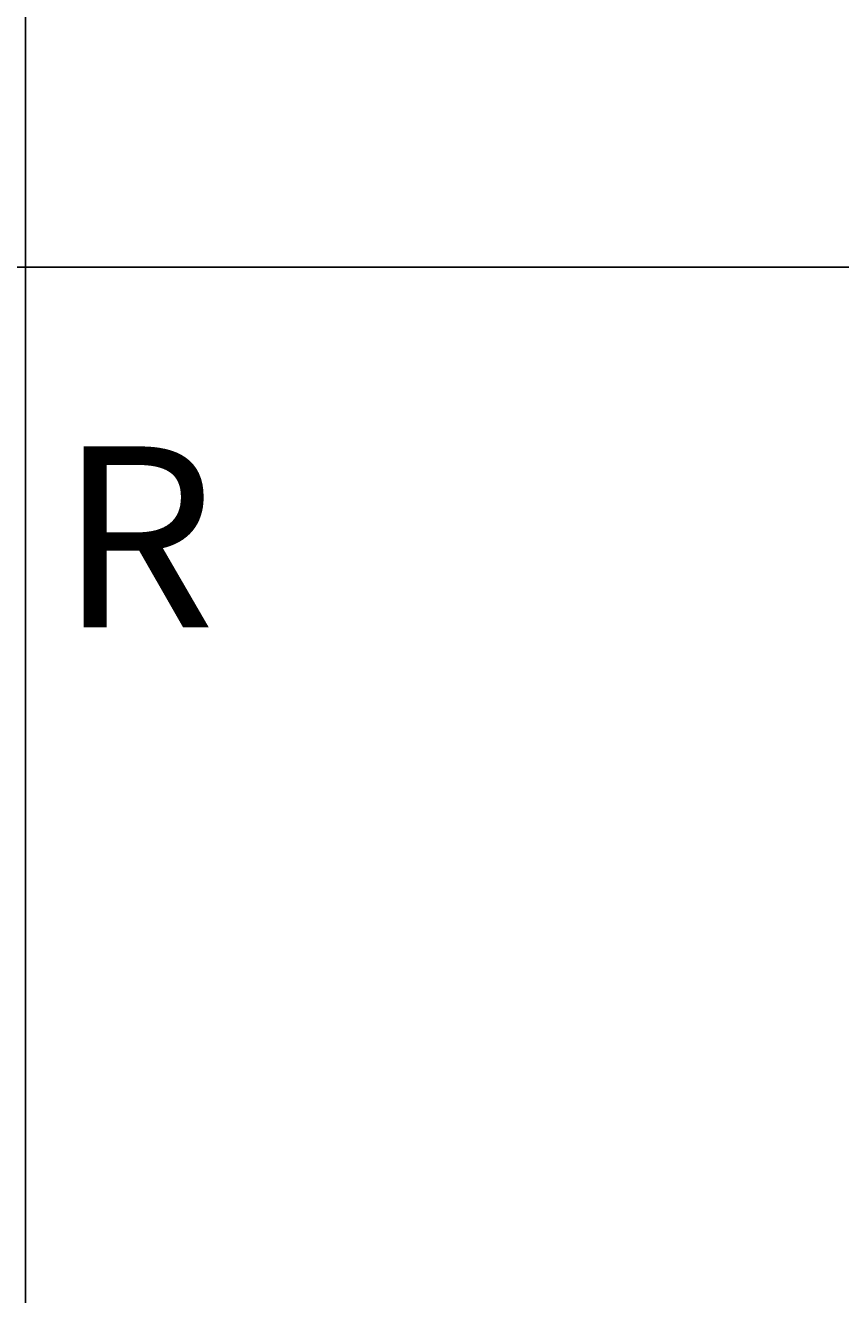
# Model space of a CAD drawing. Units: inches. Extents: x 35362 to 73946, y 43607 to 67532.
# Tile 134 of 134: x 67327 to 68321, y 57027 to 58575. Entities that reach past the tile are written whole.
import ezdxf

# ---------------------------------------------------------------- set-up
doc = ezdxf.new("R2010")
doc.units = ezdxf.units.IN
doc.header["$MEASUREMENT"] = 0
doc.layers.add('A-ANNO-DIMS', color=2, linetype='Continuous', lineweight=18)
doc.layers.add('E-ANNO-TEXT', color=5, linetype='Continuous', lineweight=18)
doc.styles.get("Standard").update_dxf_attribs({"font": 'arial.ttf'})
doc.dimstyles.get("Standard").update_dxf_attribs({"dimtxt": 0.18, "dimasz": 0.18, "dimexe": 0.18, "dimexo": 0.0625, "dimgap": 0.09, "dimtad": 0, "dimtih": 1, "dimtoh": 1, "dimdec": 4, "dimzin": 0, "dimdsep": 46, "dimtxsty": 'Standard', "dimcen": 0.09, "dimadec": 0, "dimazin": 0, "dimtfac": 1, "dimtdec": 4, "dimtofl": 0, "dimtmove": 0, "dimatfit": 3, "dimfxl": 1, "dimtolj": 1, "dimtzin": 0, "dimarcsym": 0})

# ---------------------------------------------------------------- blocks, each defined once
blk = doc.blocks.new('*D8')
at = {"layer": 'A-ANNO-DIMS', "color": 0, "lineweight": -2, "transparency": 16777216}
for p, q in [((66271.28651900003, 65771.51172800003), (73945.82566600003, 65771.51172800003)), ((73945.64566600005, 65771.33172800003), (73945.64566600005, 59737.03093663782)), ((73945.64566600005, 53702.36633900002), (73945.64566600005, 59736.66713036224)), ((72185.70816600003, 53702.18633900003), (73945.82566600003, 53702.18633900003))]:
    blk.add_line(p, q, dxfattribs=at)
at = {"layer": 'A-ANNO-DIMS', "color": 0, "transparency": 16777216}
for points in [[(73945.61566600006, 65771.33172800003), (73945.67566600005, 65771.33172800003), (73945.64566600005, 65771.51172800003)], [(73945.61566600006, 53702.36633900002), (73945.67566600005, 53702.36633900002), (73945.64566600005, 53702.18633900003)]]:
    blk.add_solid(points, dxfattribs=at)
at = {"layer": 'Defpoints', "color": 0, "transparency": 16777216}
for p in [(66271.22401900003, 65771.51172800003), (73945.64566600005, 65771.51172800003), (72185.64566600003, 53702.18633900003)]:
    blk.add_point(p, dxfattribs=at)
at = {"layer": 'A-ANNO-DIMS', "color": 0, "transparency": 16777216, "insert": (73945.64566600005, 59736.84903349999), "char_height": 0.18, "attachment_point": 5}
blk.add_mtext('\\A1;12069', dxfattribs=at)
blk = doc.blocks.new('*D10')
at = {"layer": 'A-ANNO-DIMS', "color": 0, "lineweight": -2, "transparency": 16777216}
for p, q in [((61240.96983600002, 59185.14395700003), (73945.82566600003, 59185.14395700003)), ((73945.64566600005, 59184.96395700003), (73945.64566600005, 56268.51827402935)), ((73945.64566600005, 53351.70866200003), (73945.64566600005, 56268.1543449707)), ((61240.96983600002, 53351.52866200003), (73945.82566600003, 53351.52866200003))]:
    blk.add_line(p, q, dxfattribs=at)
at = {"layer": 'A-ANNO-DIMS', "color": 0, "transparency": 16777216}
for points in [[(73945.61566600006, 59184.96395700003), (73945.67566600005, 59184.96395700003), (73945.64566600005, 59185.14395700003)], [(73945.61566600006, 53351.70866200003), (73945.67566600005, 53351.70866200003), (73945.64566600005, 53351.52866200003)]]:
    blk.add_solid(points, dxfattribs=at)
at = {"layer": 'Defpoints', "color": 0, "transparency": 16777216}
for p in [(61240.90733600002, 59185.14395700003), (61240.90733600002, 53351.52866200003), (73945.64566600005, 53351.52866200003)]:
    blk.add_point(p, dxfattribs=at)
at = {"layer": 'A-ANNO-DIMS', "color": 0, "transparency": 16777216, "insert": (73945.64566600005, 56268.33630949999), "char_height": 0.18, "attachment_point": 5}
blk.add_mtext('\\A1;5834', dxfattribs=at)
blk = doc.blocks.new('*D36')
at = {"layer": 'A-ANNO-DIMS', "color": 0, "lineweight": -2, "transparency": 16777216}
for p, q in [((68320.80826200004, 60122.34633200002), (35361.76908500003, 60122.34633200002)), ((35361.94908500003, 60122.16633200002), (35361.94908500003, 57247.82893113781)), ((35361.94908500003, 54373.12772400002), (35361.94908500003, 57247.46512486223)), ((68320.80826200004, 54372.94772400003), (35361.76908500003, 54372.94772400002))]:
    blk.add_line(p, q, dxfattribs=at)
at = {"layer": 'A-ANNO-DIMS', "color": 0, "transparency": 16777216}
for points in [[(35361.91908500003, 60122.16633200002), (35361.97908500003, 60122.16633200002), (35361.94908500003, 60122.34633200002)], [(35361.91908500003, 54373.12772400002), (35361.97908500003, 54373.12772400002), (35361.94908500003, 54372.94772400002)]]:
    blk.add_solid(points, dxfattribs=at)
at = {"layer": 'Defpoints', "color": 0, "transparency": 16777216}
for p in [(68320.87076200004, 60122.34633200002), (35361.94908500003, 54372.94772400002), (68320.87076200004, 54372.94772400003)]:
    blk.add_point(p, dxfattribs=at)
at = {"layer": 'A-ANNO-DIMS', "color": 0, "transparency": 16777216, "insert": (35361.94908500004, 57247.64702799999), "char_height": 0.18, "attachment_point": 5}
blk.add_mtext('\\A1;5749.4', dxfattribs=at)
blk = doc.blocks.new('*D47')
at = {"layer": 'A-ANNO-DIMS', "color": 0, "lineweight": -2, "transparency": 16777216}
for p, q in [((50339.58680000003, 58279.98849500002), (73945.82566600003, 58279.98849500002)), ((73945.64566600005, 58279.80849500002), (73945.64566600005, 57564.17141502935)), ((73945.64566600005, 56848.17040600003), (73945.64566600005, 57563.80748597069)), ((50339.58680000003, 56847.99040600003), (73945.82566600003, 56847.99040600003))]:
    blk.add_line(p, q, dxfattribs=at)
at = {"layer": 'A-ANNO-DIMS', "color": 0, "transparency": 16777216}
for points in [[(73945.61566600006, 58279.80849500002), (73945.67566600005, 58279.80849500002), (73945.64566600005, 58279.98849500002)], [(73945.61566600006, 56848.17040600003), (73945.67566600005, 56848.17040600003), (73945.64566600005, 56847.99040600003)]]:
    blk.add_solid(points, dxfattribs=at)
at = {"layer": 'Defpoints', "color": 0, "transparency": 16777216}
for p in [(50339.52430000002, 58279.98849500002), (50339.52430000002, 56847.99040600003), (73945.64566600005, 56847.99040600003)]:
    blk.add_point(p, dxfattribs=at)
at = {"layer": 'A-ANNO-DIMS', "color": 0, "transparency": 16777216, "insert": (73945.64566600005, 57563.98945049999), "char_height": 0.18, "attachment_point": 5}
blk.add_mtext('\\A1;1432.0', dxfattribs=at)
blk = doc.blocks.new('*D65')
at = {"layer": 'A-ANNO-DIMS', "color": 0, "lineweight": -2, "transparency": 16777216}
for p, q in [((65336.01600799999, 61293.223552), (65336.01600799999, 43606.678996)), ((67326.639741, 61293.223552), (67326.639741, 43606.678996)), ((65336.19600799999, 43606.858996), (66330.87277900206, 43606.858996)), ((67326.45974100001, 43606.858996), (66331.78296999796, 43606.858996))]:
    blk.add_line(p, q, dxfattribs=at)
at = {"layer": 'A-ANNO-DIMS', "color": 0, "transparency": 16777216}
for points in [[(65336.19600799999, 43606.888996), (65336.19600799999, 43606.828996), (65336.01600799999, 43606.858996)], [(67326.45974100001, 43606.888996), (67326.45974100001, 43606.828996), (67326.639741, 43606.858996)]]:
    blk.add_solid(points, dxfattribs=at)
at = {"layer": 'Defpoints', "color": 0, "transparency": 16777216}
for p in [(65336.01600799999, 61293.286052), (67326.639741, 61293.286052), (67326.639741, 43606.858996)]:
    blk.add_point(p, dxfattribs=at)
at = {"layer": 'A-ANNO-DIMS', "color": 0, "transparency": 16777216, "insert": (66331.32787450001, 43606.858996), "char_height": 0.18, "attachment_point": 5}
blk.add_mtext('\\A1;1990.6', dxfattribs=at)

msp = doc.modelspace()

# ---------------------------------------------------------------- texts
at = {"layer": 'E-ANNO-TEXT'}
msp.add_text('R', height=220.8659825270206, dxfattribs=at).set_placement((67367.47822977841, 57840.5564139079))

# ---------------------------------------------------------------- dimensions: what is measured, and where the dimension line sits
at = {"layer": 'A-ANNO-DIMS'}
for base, p1, p2, override, picture, middle in [((73945.64566600005, 65771.51172800003), (72185.645666, 53702.186339), (66271.224019, 65771.51172799998), {"dimdec": 0, "dimlfac": 1, "dimrnd": 0, "dimzin": 0, "dimdsep": 46, "dimlunit": 2}, '*D8', (73945.64566600005, 59736.84903349999)), ((35361.94908500003, 54372.94772400002), (68320.870762, 60122.346332), (68320.870762, 54372.947724), {"dimdec": 1, "dimlfac": 1, "dimrnd": 0, "dimzin": 0, "dimdsep": 46, "dimlunit": 2}, '*D36', (35361.94908500004, 57247.64702799999)), ((73945.64566600005, 53351.52866200003), (61240.907336, 59185.14395699999), (61240.907336, 53351.52866199999), {"dimdec": 0, "dimlfac": 1, "dimrnd": 0, "dimzin": 0, "dimdsep": 46, "dimlunit": 2}, '*D10', (73945.64566600005, 56268.33630949999)), ((73945.64566600005, 56847.99040600003), (50339.5243, 58279.988495), (50339.5243, 56847.99040599999), {"dimdec": 1, "dimlfac": 1, "dimrnd": 0, "dimzin": 0, "dimdsep": 46, "dimlunit": 2}, '*D47', (73945.64566600005, 57563.98945049999))]:
    dim = msp.add_linear_dim(base=base, p1=p1, p2=p2, angle=90, dimstyle='Standard', override=override, dxfattribs=at)
    dim.commit()
    dim.dimension.update_dxf_attribs({"geometry": picture, "text_midpoint": middle})
dim = msp.add_linear_dim(base=(67326.639741, 43606.858996), p1=(65336.01600799999, 61293.286052), p2=(67326.639741, 61293.286052), dimstyle='Standard', override={"dimdec": 1, "dimlfac": 1, "dimrnd": 0, "dimzin": 0, "dimdsep": 46, "dimlunit": 2}, dxfattribs=at)
dim.commit()
dim.dimension.update_dxf_attribs({"geometry": '*D65', "text_midpoint": (66331.32787450001, 43606.858996)})

doc.saveas('drawing.dxf')
